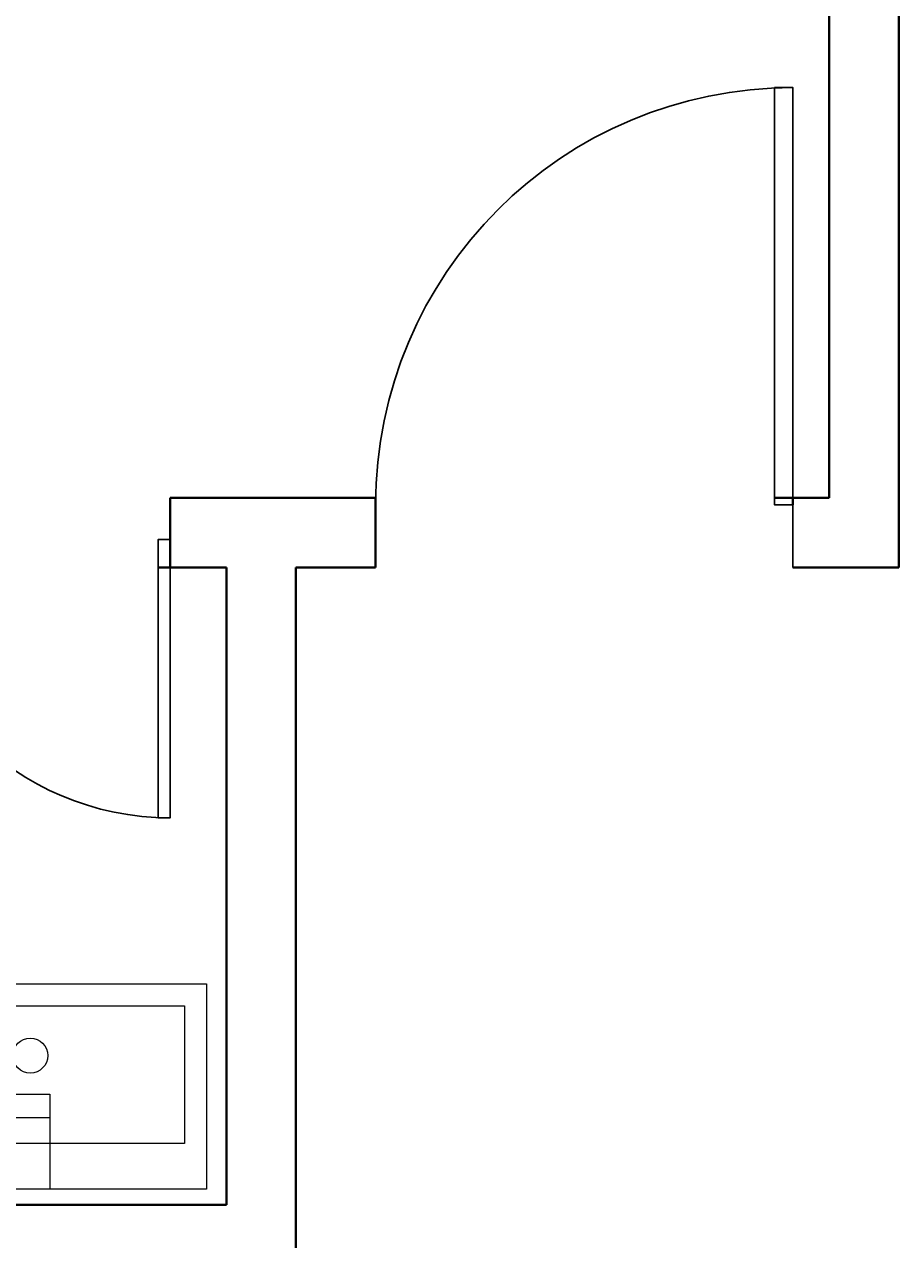
# Model space of a CAD drawing. Units: inches. Extents: x -46 to 1145, y -527 to 760.
# Tile 42 of 57: x 114 to 190, y 443 to 547. Entities that reach past the tile are written whole.
import ezdxf

# ---------------------------------------------------------------- set-up
doc = ezdxf.new("R2010")
doc.units = ezdxf.units.IN
doc.header["$MEASUREMENT"] = 0
for name, color, linetype, lineweight in [('A-ANNO-DIMS', 2, 'Continuous', 18), ('A-FLOR-FIXT', 9, 'Continuous', 18), ('DOORS', 3, 'Continuous', 25), ('WALLS', 4, 'Continuous', 40)]:
    doc.layers.add(name, color=color, linetype=linetype, lineweight=lineweight)
doc.styles.get("Standard").update_dxf_attribs({"font": 'arial.ttf'})
doc.dimstyles.get("Standard").update_dxf_attribs({"dimtxt": 0.18, "dimasz": 0.18, "dimexe": 0.18, "dimexo": 0.0625, "dimgap": 0.09, "dimtad": 0, "dimtih": 1, "dimtoh": 1, "dimdec": 0, "dimzin": 0, "dimdsep": 46, "dimlunit": 3, "dimtxsty": 'Standard', "dimcen": 0.09, "dimadec": 0, "dimazin": 0, "dimtfac": 1, "dimtdec": 0, "dimtofl": 0, "dimtmove": 0, "dimatfit": 3, "dimfxl": 1, "dimtolj": 1, "dimtzin": 0, "dimarcsym": 0})

# ---------------------------------------------------------------- blocks, each defined once
blk = doc.blocks.new('*U2')
for p, q in [((0, 0), (0, -6)), ((40, 0), (40, -6))]:
    blk.add_line(p, q)
blk.add_lwpolyline([(0, 0), (0, 40), (1.75, 40), (1.75, 0)], close=True)
blk.add_arc((0, 0), 40, 0, 90)
blk = doc.blocks.new('LAVATORY-RECT')
blk.add_line((14.01, 6.17), (17.08, 6.17))
for points in [[(30.61, 0), (0, 0), (0, 17.7), (30.61, 17.7)], [(28.7, 3.94), (1.97, 3.94), (1.97, 15.81), (28.7, 15.81)], [(17.08, 0), (14.01, 0), (14.01, 8.17), (17.08, 8.17)]]:
    blk.add_lwpolyline(points, close=True)
blk.add_circle((15.39, 11.51), 1.51)
blk = doc.blocks.new('*D685')
at = {"layer": 'A-ANNO-DIMS', "color": 0, "lineweight": -2, "transparency": 16777216}
for p, q in [((183.5, 700.89), (-46.22, 700.89)), ((-46.04, 700.71), (-46.04, 116.39)), ((-46.04, -468.3), (-46.04, 116.02)), ((12.5, -468.48), (-46.22, -468.48))]:
    blk.add_line(p, q, dxfattribs=at)
at = {"layer": 'A-ANNO-DIMS', "color": 0, "transparency": 16777216}
for points in [[(-46.07, 700.71), (-46.01, 700.71), (-46.04, 700.89)], [(-46.07, -468.3), (-46.01, -468.3), (-46.04, -468.48)]]:
    blk.add_solid(points, dxfattribs=at)
at = {"layer": 'Defpoints', "color": 0, "transparency": 16777216}
for p in [(-46.04, 700.89), (183.56, 700.89), (12.56, -468.48)]:
    blk.add_point(p, dxfattribs=at)
at = {"layer": 'A-ANNO-DIMS', "color": 0, "transparency": 16777216, "insert": (-46.04, 116.2), "char_height": 0.18, "attachment_point": 5}
blk.add_mtext('\\A1;1169.4', dxfattribs=at)

msp = doc.modelspace()

# ---------------------------------------------------------------- linework, layer by layer
at = {"layer": 'WALLS'}
for p, q in [((189.5637, 659.5176), (189.5637, 500.5176)), ((183.5637, 650.5176), (183.5637, 506.5176)), ((126.7169, 506.5176), (126.7169, 500.5176)), ((144.4431, 506.5176), (126.7169, 506.5176)), ((144.4381, 500.5176), (144.4381, 506.5176)), ((183.5637, 506.5176), (178.8631, 506.5176)), ((180.4381, 505.9176), (180.4381, 506.5176)), ((131.5637, 500.5176), (125.6669, 500.5176)), ((131.5637, 445.5176), (131.5637, 500.5176)), ((137.5637, 439.5176), (137.5637, 500.5176)), ((144.4381, 500.5176), (137.5637, 500.5176)), ((189.5637, 500.5176), (180.4381, 500.5176)), ((131.5637, 445.5176), (21.5637, 445.5176))]:
    msp.add_line(p, q, dxfattribs=at)

# ---------------------------------------------------------------- block references
at = {"layer": 'A-FLOR-FIXT'}
msp.add_blockref('LAVATORY-RECT', (99.252, 446.889), dxfattribs=at)
at = {"layer": 'DOORS', "xscale": -0.9, "yscale": 0.9, "zscale": 0.9}
msp.add_blockref('*U2', (180.4381, 505.9176), dxfattribs=at)
at = {"layer": 'DOORS', "xscale": 0.6, "yscale": 0.6, "zscale": 0.6, "rotation": 180}
msp.add_blockref('*U2', (126.7169, 502.9176), dxfattribs=at)

# ---------------------------------------------------------------- dimensions: what is measured, and where the dimension line sits
at = {"layer": 'A-ANNO-DIMS'}
dim = msp.add_linear_dim(base=(-46.0363, 700.8886), p1=(12.5637, -468.4824), p2=(183.5637, 700.8886), angle=90, dimstyle='Standard', override={"dimdec": 1, "dimlfac": 1, "dimrnd": 0, "dimzin": 0, "dimdsep": 46, "dimlunit": 2}, dxfattribs=at)
dim.commit()
dim.dimension.update_dxf_attribs({"geometry": '*D685', "text_midpoint": (-46.0363, 116.2031)})

doc.saveas('drawing.dxf')
